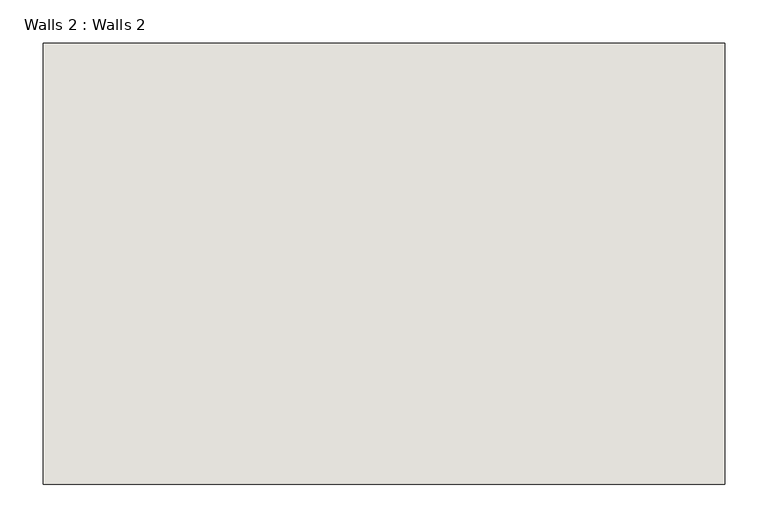
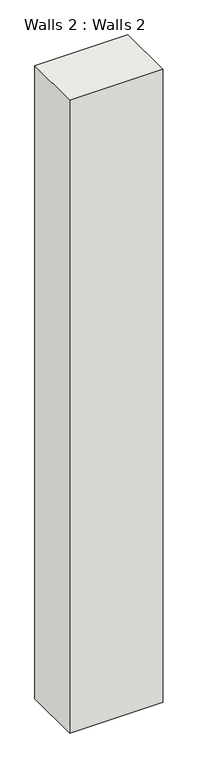
"""IFC4 building model written with IfcOpenShell, lengths in millimetres: wall geometry, Walls 2 : Walls 2."""

from ifc_helpers import new_model, si_unit, origin, origin_with_axes, place, context, project, spatial, polyline, outline, extrude, source, transform, mapped, element, save


def walls_2_walls_2_e7feafe1(model_context):
    return source(origin(), model_context, "Body", "SweptSolid", [
        extrude(outline(polyline([(-17716.4633774, -20639.6232009), (-18502.2383357, -20639.6232009), (-18502.2383357, -20130.9210337), (-17716.4633774, -20130.9210337), (-17716.4633774, -20639.6232009)])), origin_with_axes(), (0.0, 0.0, 1.0), 5648.0),
    ])


if __name__ == "__main__":
    model = new_model("IFC4")
    model_context = context("Model", 3, world=origin())
    ifc_project = project(units=[si_unit("LENGTHUNIT", "METRE", prefix="MILLI")], contexts=[model_context])
    site = spatial("IfcSite", under=ifc_project)
    building = spatial("IfcBuilding", under=site)
    placement = place(None, origin())
    walls_2_walls_2_shape = walls_2_walls_2_e7feafe1(model_context)
    element("IfcWall", 1, ObjectType="Walls 2 : Walls 2", at=placement, inside=building, context=model_context, shape_type="MappedRepresentation", body=[
        mapped(walls_2_walls_2_shape, transform((0.0, 0.0, 0.0), x_axis=(1.0, 0.0, 0.0), y_axis=(0.0, 1.0, 0.0), z_axis=(0.0, 0.0, 1.0))),
    ])
    save(model, "model.ifc")

# Revit data of these elements
# Element 1 (IfcWall, "Walls 2 : Walls 2")
#   Materials on its faces: "Default Wall"
# Materials
#   "Default Wall": colour RGB 80 80 80, transparency 0
